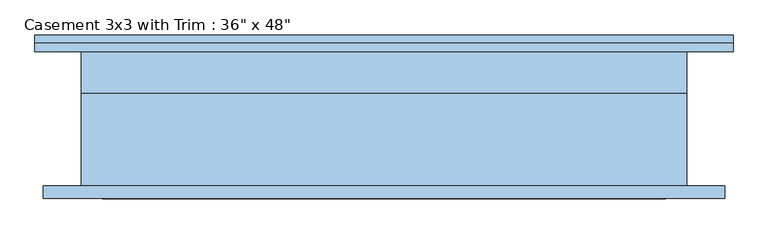
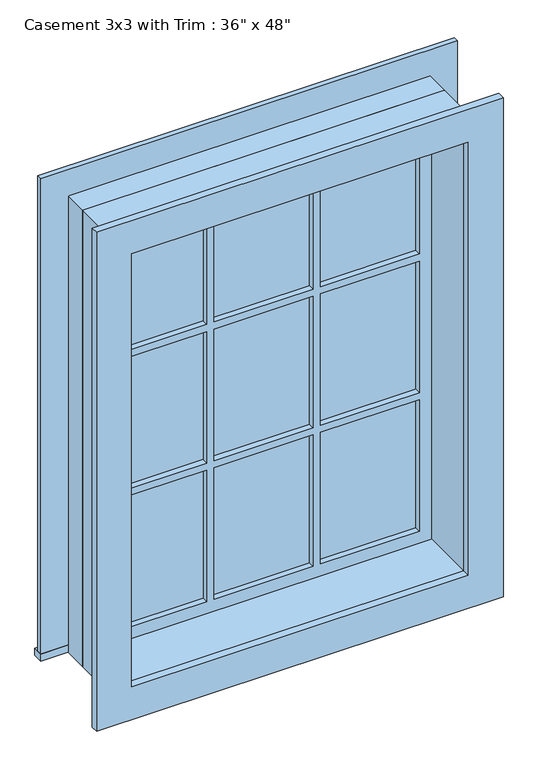
"""IFC4 building model written with IfcOpenShell, lengths in millimetres: window geometry."""

from ifc_helpers import new_model, si_unit, frame, origin, place, context, project, spatial, polyline, outline, extrude, source, transform, mapped, element, save


def window_29c06734(model_context):
    return source(origin(), model_context, "Body", "SweptSolid", [
        extrude(outline(polyline([(-527.05, 127.0), (527.05, 127.0), (527.05, 101.6), (-527.05, 101.6), (-527.05, 127.0)])), frame((0.0, 0.0, 914.4), z_axis=(0.0, 0.0, 1.0), x_axis=(1.0, 0.0, 0.0)), (0.0, 0.0, 1.0), 19.05),
        extrude(outline(polyline([(2114.55, -438.15), (2114.55, 438.15), (933.45, 438.15), (933.45, 527.05), (2203.45, 527.05), (2203.45, -527.05), (933.45, -527.05), (933.45, -438.15), (2114.55, -438.15)])), frame((0.0, 101.6, 0.0), z_axis=(0.0, 1.0, 0.0), x_axis=(0.0, 0.0, 1.0)), (0.0, 0.0, 1.0), 12.7),
        extrude(outline(polyline([(143.9333333, 66.675), (393.7, 66.675), (393.7, 53.975), (143.9333333, 53.975), (143.9333333, 66.675)])), frame((0.0, 0.0, 1718.7333333), z_axis=(0.0, 0.0, 1.0), x_axis=(1.0, 0.0, 0.0)), (0.0, 0.0, 1.0), 351.3666667),
        extrude(outline(polyline([(-124.8833333, 66.675), (124.8833333, 66.675), (124.8833333, 53.975), (-124.8833333, 53.975), (-124.8833333, 66.675)])), frame((0.0, 0.0, 1718.7333333), z_axis=(0.0, 0.0, 1.0), x_axis=(1.0, 0.0, 0.0)), (0.0, 0.0, 1.0), 351.3666667),
        extrude(outline(polyline([(-393.7, 66.675), (-143.9333333, 66.675), (-143.9333333, 53.975), (-393.7, 53.975), (-393.7, 66.675)])), frame((0.0, 0.0, 1718.7333333), z_axis=(0.0, 0.0, 1.0), x_axis=(1.0, 0.0, 0.0)), (0.0, 0.0, 1.0), 351.3666667),
        extrude(outline(polyline([(-393.7, 66.675), (-143.9333333, 66.675), (-143.9333333, 53.975), (-393.7, 53.975), (-393.7, 66.675)])), frame((0.0, 0.0, 1348.3166667), z_axis=(0.0, 0.0, 1.0), x_axis=(1.0, 0.0, 0.0)), (0.0, 0.0, 1.0), 351.3666667),
        extrude(outline(polyline([(-124.8833333, 66.675), (124.8833333, 66.675), (124.8833333, 53.975), (-124.8833333, 53.975), (-124.8833333, 66.675)])), frame((0.0, 0.0, 1348.3166667), z_axis=(0.0, 0.0, 1.0), x_axis=(1.0, 0.0, 0.0)), (0.0, 0.0, 1.0), 351.3666667),
        extrude(outline(polyline([(143.9333333, 66.675), (393.7, 66.675), (393.7, 53.975), (143.9333333, 53.975), (143.9333333, 66.675)])), frame((0.0, 0.0, 1348.3166667), z_axis=(0.0, 0.0, 1.0), x_axis=(1.0, 0.0, 0.0)), (0.0, 0.0, 1.0), 351.3666667),
        extrude(outline(polyline([(143.9333333, 66.675), (393.7, 66.675), (393.7, 53.975), (143.9333333, 53.975), (143.9333333, 66.675)])), frame((0.0, 0.0, 977.9), z_axis=(0.0, 0.0, 1.0), x_axis=(1.0, 0.0, 0.0)), (0.0, 0.0, 1.0), 351.3666667),
        extrude(outline(polyline([(-124.8833333, 66.675), (124.8833333, 66.675), (124.8833333, 53.975), (-124.8833333, 53.975), (-124.8833333, 66.675)])), frame((0.0, 0.0, 977.9), z_axis=(0.0, 0.0, 1.0), x_axis=(1.0, 0.0, 0.0)), (0.0, 0.0, 1.0), 351.3666667),
        extrude(outline(polyline([(-393.7, 66.675), (-143.9333333, 66.675), (-143.9333333, 53.975), (-393.7, 53.975), (-393.7, 66.675)])), frame((0.0, 0.0, 977.9), z_axis=(0.0, 0.0, 1.0), x_axis=(1.0, 0.0, 0.0)), (0.0, 0.0, 1.0), 351.3666667),
        extrude(outline(polyline([(2190.75, 514.35), (2190.75, -514.35), (857.25, -514.35), (857.25, 514.35), (2190.75, 514.35)]), holes=[polyline([(2101.85, 425.45), (946.15, 425.45), (946.15, -425.45), (2101.85, -425.45), (2101.85, 425.45)])]), frame((0.0, -120.65, 0.0), z_axis=(0.0, 1.0, 0.0), x_axis=(0.0, 0.0, 1.0)), (0.0, 0.0, 1.0), 19.05),
        extrude(outline(polyline([(2114.55, -438.15), (933.45, -438.15), (933.45, 438.15), (2114.55, 438.15), (2114.55, -438.15)]), holes=[polyline([(2070.1, -143.9333333), (1718.7333333, -143.9333333), (1718.7333333, -393.7), (2070.1, -393.7), (2070.1, -143.9333333)]), polyline([(1699.6833333, -143.9333333), (1348.3166667, -143.9333333), (1348.3166667, -393.7), (1699.6833333, -393.7), (1699.6833333, -143.9333333)]), polyline([(1329.2666667, -143.9333333), (977.9, -143.9333333), (977.9, -393.7), (1329.2666667, -393.7), (1329.2666667, -143.9333333)]), polyline([(2070.1, 124.8833333), (1718.7333333, 124.8833333), (1718.7333333, -124.8833333), (2070.1, -124.8833333), (2070.1, 124.8833333)]), polyline([(1699.6833333, 124.8833333), (1348.3166667, 124.8833333), (1348.3166667, -124.8833333), (1699.6833333, -124.8833333), (1699.6833333, 124.8833333)]), polyline([(1329.2666667, 124.8833333), (977.9, 124.8833333), (977.9, -124.8833333), (1329.2666667, -124.8833333), (1329.2666667, 124.8833333)]), polyline([(2070.1, 393.7), (1718.7333333, 393.7), (1718.7333333, 143.9333333), (2070.1, 143.9333333), (2070.1, 393.7)]), polyline([(1699.6833333, 393.7), (1348.3166667, 393.7), (1348.3166667, 143.9333333), (1699.6833333, 143.9333333), (1699.6833333, 393.7)]), polyline([(1329.2666667, 393.7), (977.9, 393.7), (977.9, 143.9333333), (1329.2666667, 143.9333333), (1329.2666667, 393.7)])]), frame((0.0, 38.1, 0.0), z_axis=(0.0, 1.0, 0.0), x_axis=(0.0, 0.0, 1.0)), (0.0, 0.0, 1.0), 44.45),
        extrude(outline(polyline([(2133.6, -457.2), (914.4, -457.2), (914.4, 457.2), (2133.6, 457.2), (2133.6, -457.2)]), holes=[polyline([(2101.85, -425.45), (2101.85, 425.45), (946.15, 425.45), (946.15, -425.45), (2101.85, -425.45)])]), frame((0.0, -101.6, 0.0), z_axis=(0.0, 1.0, 0.0), x_axis=(0.0, 0.0, 1.0)), (0.0, 0.0, 1.0), 139.7),
        extrude(outline(polyline([(2133.6, 457.2), (2133.6, -457.2), (914.4, -457.2), (914.4, 457.2), (2133.6, 457.2)]), holes=[polyline([(2114.55, 438.15), (933.45, 438.15), (933.45, -438.15), (2114.55, -438.15), (2114.55, 438.15)])]), frame((0.0, 38.1, 0.0), z_axis=(0.0, 1.0, 0.0), x_axis=(0.0, 0.0, 1.0)), (0.0, 0.0, 1.0), 63.5),
    ])


if __name__ == "__main__":
    model = new_model("IFC4")
    model_context = context("Model", 3, world=origin())
    ifc_project = project(units=[si_unit("LENGTHUNIT", "METRE", prefix="MILLI")], contexts=[model_context])
    site = spatial("IfcSite", under=ifc_project)
    building = spatial("IfcBuilding", under=site)
    placement = place(None, origin())
    window_shape = window_29c06734(model_context)
    element("IfcWindow", 1, ObjectType="Casement 3x3 with Trim : 36\" x 48\"", at=placement, inside=building, context=model_context, shape_type="MappedRepresentation", body=[
        mapped(window_shape, transform((0.0, 0.0, 0.0), x_axis=(1.0, 0.0, 0.0), y_axis=(0.0, 1.0, 0.0), z_axis=(0.0, 0.0, 1.0))),
    ])
    save(model, "model.ifc")

# Revit data of these elements
# Type "Casement 3x3 with Trim : 36\" x 48\""
#   Type Mark = "10"
#   Construction Type Id = "GSP4R"
#   Assembly Code = "B2020100"
#   Analytic Construction = "1/8 in Pilkington single glazing"
#   Visual Light Transmittance = 0.9
#   Solar Heat Gain Coefficient = 0.78
#   Heat Transfer Coefficient (U) = 0.6496 BTU/(h·ft²·°F)
#   Height = 4' - 0"
#   Default Sill Height = 3' - 0"
#   Trim Projection - Ext. = 0' - 0 1/2"
#   Trim Projection - Int. = 0' - 0 3/4"
#   Trim Width - Exterior = 0' - 3 1/2"
#   Trim Width - Interior = 0' - 3 1/2"
#   Width = 3' - 0"
#   Window Inset = 0' - 0 3/4"
#   Define Thermal Properties by = 1
#   Glass Pane Material = Glass
#   Sash Material = Sash
#   Trim Exterior Material = Trim
#   Trim Interior Material = Trim
#   Wall Closure = (empty or 0)
# Element 1 (IfcWindow, "Casement 3x3 with Trim : 36\" x 48\"")
#   Materials on its faces: "Sash", "Glass", "Trim"
# Materials
#   "Glass": class "Glass", colour RGB 0 128 192, transparency 0.75, Description = "Soda Lime Glass", Cost = 0
#   "Sash": class "Wood", colour RGB 224 178 126, transparency 0
#   "Trim": class "Wood", colour RGB 224 178 126, transparency 0
